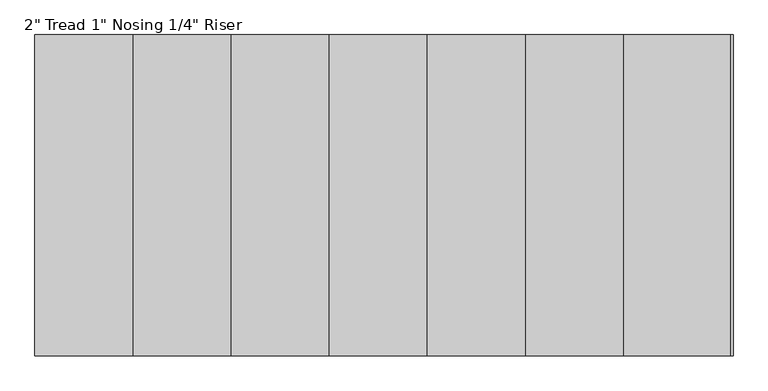
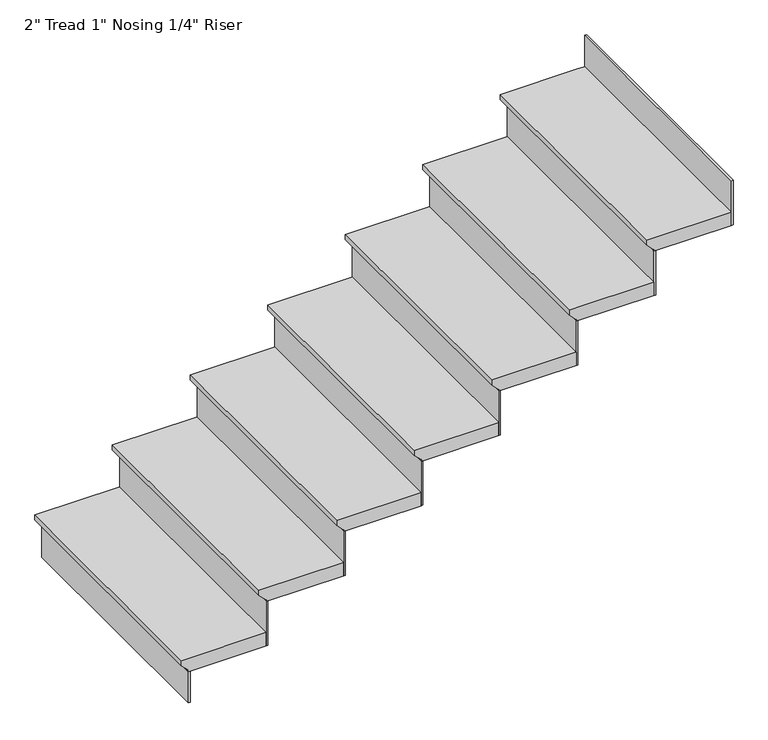
"""IFC4 building model written with IfcOpenShell, lengths in millimetres: stair flight geometry."""

from ifc_helpers import new_model, si_unit, origin, place, context, project, spatial, faceted_brep, source, transform, mapped, element, save


def stair_flight_c73b5a8b(model_context):
    return source(origin(), model_context, "Body", "Brep", [
        faceted_brep([(-3636.7866603, -3450.3331121, 150.2833333), (-3636.7866603, -3450.3331121, 169.3333333), (-3636.7866603, -2535.9331121, 169.3333333), (-3636.7866603, -2535.9331121, 150.2833333), (-3611.3866603, -3450.3331121, 124.8833333), (-3611.3866603, -2535.9331121, 124.8833333), (-3331.9866603, -3450.3331121, 169.3333333), (-3331.9866603, -2535.9331121, 169.3333333), (-3611.3866603, -2535.9331121, 118.5333333), (-3331.9866603, -2535.9331121, 118.5333333), (-3331.9866603, -3450.3331121, 118.5333333), (-3611.3866603, -3450.3331121, 118.5333333)], [[[0, 1, 2, 3]], [[4, 0, 3, 5]], [[2, 1, 6, 7]], [[8, 9, 10, 11]], [[2, 7, 9, 8, 5, 3]], [[8, 11, 4, 5]], [[6, 1, 0, 4, 11, 10]], [[7, 6, 10, 9]]]),
        faceted_brep([(-3611.3866603, -3450.3331121, 118.5333333), (-3611.3866603, -3450.3331121, 0.0), (-3605.0366603, -3450.3331121, 0.0), (-3605.0366603, -3450.3331121, 118.5333333), (-3611.3866603, -2535.9331121, 118.5333333), (-3605.0366603, -2535.9331121, 118.5333333), (-3605.0366603, -2535.9331121, 0.0), (-3611.3866603, -2535.9331121, 0.0)], [[[0, 1, 2, 3]], [[4, 5, 6, 7]], [[1, 0, 4, 7]], [[2, 1, 7, 6]], [[3, 2, 6, 5]], [[0, 3, 5, 4]]]),
        faceted_brep([(-3331.9866603, -3450.3331121, 287.8666667), (-3331.9866603, -3450.3331121, 118.5333333), (-3325.6366603, -3450.3331121, 118.5333333), (-3325.6366603, -3450.3331121, 287.8666667), (-3331.9866603, -2535.9331121, 287.8666667), (-3325.6366603, -2535.9331121, 287.8666667), (-3325.6366603, -2535.9331121, 118.5333333), (-3331.9866603, -2535.9331121, 118.5333333)], [[[0, 1, 2, 3]], [[4, 5, 6, 7]], [[1, 0, 4, 7]], [[2, 1, 7, 6]], [[3, 2, 6, 5]], [[0, 3, 5, 4]]]),
        faceted_brep([(-3357.3866603, -2535.9331121, 338.6666667), (-3357.3866603, -3450.3331121, 338.6666667), (-3052.5866603, -3450.3331121, 338.6666667), (-3052.5866603, -2535.9331121, 338.6666667), (-3331.9866603, -2535.9331121, 287.8666667), (-3052.5866603, -2535.9331121, 287.8666667), (-3052.5866603, -3450.3331121, 287.8666667), (-3331.9866603, -3450.3331121, 287.8666667), (-3331.9866603, -2535.9331121, 294.2166667), (-3357.3866603, -2535.9331121, 319.6166667), (-3331.9866603, -3450.3331121, 294.2166667), (-3357.3866603, -3450.3331121, 319.6166667)], [[[0, 1, 2, 3]], [[4, 5, 6, 7]], [[0, 3, 5, 4, 8, 9]], [[4, 7, 10, 8]], [[2, 1, 11, 10, 7, 6]], [[3, 2, 6, 5]], [[11, 1, 0, 9]], [[10, 11, 9, 8]]]),
        faceted_brep([(-3052.5866603, -3450.3331121, 457.2), (-3052.5866603, -3450.3331121, 287.8666667), (-3046.2366603, -3450.3331121, 287.8666667), (-3046.2366603, -3450.3331121, 457.2), (-3052.5866603, -2535.9331121, 457.2), (-3046.2366603, -2535.9331121, 457.2), (-3046.2366603, -2535.9331121, 287.8666667), (-3052.5866603, -2535.9331121, 287.8666667)], [[[0, 1, 2, 3]], [[4, 5, 6, 7]], [[1, 0, 4, 7]], [[2, 1, 7, 6]], [[3, 2, 6, 5]], [[0, 3, 5, 4]]]),
        faceted_brep([(-3077.9866603, -2535.9331121, 508.0), (-3077.9866603, -3450.3331121, 508.0), (-2773.1866603, -3450.3331121, 508.0), (-2773.1866603, -2535.9331121, 508.0), (-3052.5866603, -2535.9331121, 457.2), (-2773.1866603, -2535.9331121, 457.2), (-2773.1866603, -3450.3331121, 457.2), (-3052.5866603, -3450.3331121, 457.2), (-3052.5866603, -2535.9331121, 463.55), (-3077.9866603, -2535.9331121, 488.95), (-3052.5866603, -3450.3331121, 463.55), (-3077.9866603, -3450.3331121, 488.95)], [[[0, 1, 2, 3]], [[4, 5, 6, 7]], [[0, 3, 5, 4, 8, 9]], [[4, 7, 10, 8]], [[2, 1, 11, 10, 7, 6]], [[3, 2, 6, 5]], [[11, 1, 0, 9]], [[10, 11, 9, 8]]]),
        faceted_brep([(-2773.1866603, -3450.3331121, 626.5333333), (-2773.1866603, -3450.3331121, 457.2), (-2766.8366603, -3450.3331121, 457.2), (-2766.8366603, -3450.3331121, 626.5333333), (-2773.1866603, -2535.9331121, 626.5333333), (-2766.8366603, -2535.9331121, 626.5333333), (-2766.8366603, -2535.9331121, 457.2), (-2773.1866603, -2535.9331121, 457.2)], [[[0, 1, 2, 3]], [[4, 5, 6, 7]], [[1, 0, 4, 7]], [[2, 1, 7, 6]], [[3, 2, 6, 5]], [[0, 3, 5, 4]]]),
        faceted_brep([(-2798.5866603, -2535.9331121, 677.3333333), (-2798.5866603, -3450.3331121, 677.3333333), (-2493.7866603, -3450.3331121, 677.3333333), (-2493.7866603, -2535.9331121, 677.3333333), (-2773.1866603, -2535.9331121, 626.5333333), (-2493.7866603, -2535.9331121, 626.5333333), (-2493.7866603, -3450.3331121, 626.5333333), (-2773.1866603, -3450.3331121, 626.5333333), (-2773.1866603, -2535.9331121, 632.8833333), (-2798.5866603, -2535.9331121, 658.2833333), (-2773.1866603, -3450.3331121, 632.8833333), (-2798.5866603, -3450.3331121, 658.2833333)], [[[0, 1, 2, 3]], [[4, 5, 6, 7]], [[0, 3, 5, 4, 8, 9]], [[4, 7, 10, 8]], [[2, 1, 11, 10, 7, 6]], [[3, 2, 6, 5]], [[11, 1, 0, 9]], [[10, 11, 9, 8]]]),
        faceted_brep([(-2493.7866603, -3450.3331121, 795.8666667), (-2493.7866603, -3450.3331121, 626.5333333), (-2487.4366603, -3450.3331121, 626.5333333), (-2487.4366603, -3450.3331121, 795.8666667), (-2493.7866603, -2535.9331121, 795.8666667), (-2487.4366603, -2535.9331121, 795.8666667), (-2487.4366603, -2535.9331121, 626.5333333), (-2493.7866603, -2535.9331121, 626.5333333)], [[[0, 1, 2, 3]], [[4, 5, 6, 7]], [[1, 0, 4, 7]], [[2, 1, 7, 6]], [[3, 2, 6, 5]], [[0, 3, 5, 4]]]),
        faceted_brep([(-2519.1866603, -2535.9331121, 846.6666667), (-2519.1866603, -3450.3331121, 846.6666667), (-2214.3866603, -3450.3331121, 846.6666667), (-2214.3866603, -2535.9331121, 846.6666667), (-2493.7866603, -2535.9331121, 795.8666667), (-2214.3866603, -2535.9331121, 795.8666667), (-2214.3866603, -3450.3331121, 795.8666667), (-2493.7866603, -3450.3331121, 795.8666667), (-2493.7866603, -2535.9331121, 802.2166667), (-2519.1866603, -2535.9331121, 827.6166667), (-2493.7866603, -3450.3331121, 802.2166667), (-2519.1866603, -3450.3331121, 827.6166667)], [[[0, 1, 2, 3]], [[4, 5, 6, 7]], [[0, 3, 5, 4, 8, 9]], [[4, 7, 10, 8]], [[2, 1, 11, 10, 7, 6]], [[3, 2, 6, 5]], [[11, 1, 0, 9]], [[10, 11, 9, 8]]]),
        faceted_brep([(-2214.3866603, -3450.3331121, 965.2), (-2214.3866603, -3450.3331121, 795.8666667), (-2208.0366603, -3450.3331121, 795.8666667), (-2208.0366603, -3450.3331121, 965.2), (-2214.3866603, -2535.9331121, 965.2), (-2208.0366603, -2535.9331121, 965.2), (-2208.0366603, -2535.9331121, 795.8666667), (-2214.3866603, -2535.9331121, 795.8666667)], [[[0, 1, 2, 3]], [[4, 5, 6, 7]], [[1, 0, 4, 7]], [[2, 1, 7, 6]], [[3, 2, 6, 5]], [[0, 3, 5, 4]]]),
        faceted_brep([(-2239.7866603, -2535.9331121, 1016.0), (-2239.7866603, -3450.3331121, 1016.0), (-1934.9866603, -3450.3331121, 1016.0), (-1934.9866603, -2535.9331121, 1016.0), (-2214.3866603, -2535.9331121, 965.2), (-1934.9866603, -2535.9331121, 965.2), (-1934.9866603, -3450.3331121, 965.2), (-2214.3866603, -3450.3331121, 965.2), (-2214.3866603, -2535.9331121, 971.55), (-2239.7866603, -2535.9331121, 996.95), (-2214.3866603, -3450.3331121, 971.55), (-2239.7866603, -3450.3331121, 996.95)], [[[0, 1, 2, 3]], [[4, 5, 6, 7]], [[0, 3, 5, 4, 8, 9]], [[4, 7, 10, 8]], [[2, 1, 11, 10, 7, 6]], [[3, 2, 6, 5]], [[11, 1, 0, 9]], [[10, 11, 9, 8]]]),
        faceted_brep([(-1655.5866603, -3450.3331121, 1303.8666667), (-1655.5866603, -3450.3331121, 1134.5333333), (-1649.2366603, -3450.3331121, 1134.5333333), (-1649.2366603, -3450.3331121, 1303.8666667), (-1655.5866603, -2535.9331121, 1303.8666667), (-1649.2366603, -2535.9331121, 1303.8666667), (-1649.2366603, -2535.9331121, 1134.5333333), (-1655.5866603, -2535.9331121, 1134.5333333)], [[[0, 1, 2, 3]], [[4, 5, 6, 7]], [[1, 0, 4, 7]], [[2, 1, 7, 6]], [[3, 2, 6, 5]], [[0, 3, 5, 4]]]),
        faceted_brep([(-1934.9866603, -3450.3331121, 1134.5333333), (-1934.9866603, -3450.3331121, 965.2), (-1928.6366603, -3450.3331121, 965.2), (-1928.6366603, -3450.3331121, 1134.5333333), (-1934.9866603, -2535.9331121, 1134.5333333), (-1928.6366603, -2535.9331121, 1134.5333333), (-1928.6366603, -2535.9331121, 965.2), (-1934.9866603, -2535.9331121, 965.2)], [[[0, 1, 2, 3]], [[4, 5, 6, 7]], [[1, 0, 4, 7]], [[2, 1, 7, 6]], [[3, 2, 6, 5]], [[0, 3, 5, 4]]]),
        faceted_brep([(-1655.5866603, -2535.9331121, 1185.3333333), (-1680.9866603, -2535.9331121, 1185.3333333), (-1960.3866603, -2535.9331121, 1185.3333333), (-1960.3866603, -3450.3331121, 1185.3333333), (-1655.5866603, -3450.3331121, 1185.3333333), (-1680.9866603, -2535.9331121, 1134.5333333), (-1655.5866603, -2535.9331121, 1134.5333333), (-1655.5866603, -3450.3331121, 1134.5333333), (-1934.9866603, -3450.3331121, 1134.5333333), (-1934.9866603, -2535.9331121, 1134.5333333), (-1934.9866603, -2535.9331121, 1140.8833333), (-1960.3866603, -2535.9331121, 1166.2833333), (-1934.9866603, -3450.3331121, 1140.8833333), (-1960.3866603, -3450.3331121, 1166.2833333)], [[[0, 1, 2, 3, 4]], [[5, 6, 7, 8, 9]], [[1, 0, 6, 5]], [[2, 1, 5, 9, 10, 11]], [[9, 8, 12, 10]], [[4, 3, 13, 12, 8, 7]], [[0, 4, 7, 6]], [[13, 3, 2, 11]], [[12, 13, 11, 10]]]),
    ])


if __name__ == "__main__":
    model = new_model("IFC4")
    model_context = context("Model", 3, world=origin())
    ifc_project = project(units=[si_unit("LENGTHUNIT", "METRE", prefix="MILLI")], contexts=[model_context])
    site = spatial("IfcSite", under=ifc_project)
    building = spatial("IfcBuilding", under=site)
    placement = place(None, origin())
    stair_flight_shape = stair_flight_c73b5a8b(model_context)
    element("IfcStairFlight", 1, ObjectType="2\" Tread 1\" Nosing 1/4\" Riser", at=placement, inside=building, context=model_context, shape_type="MappedRepresentation", body=[
        mapped(stair_flight_shape, transform((0.0, 0.0, 0.0), x_axis=(1.0, 0.0, 0.0), y_axis=(0.0, 1.0, 0.0), z_axis=(0.0, 0.0, 1.0))),
    ])
    save(model, "model.ifc")
